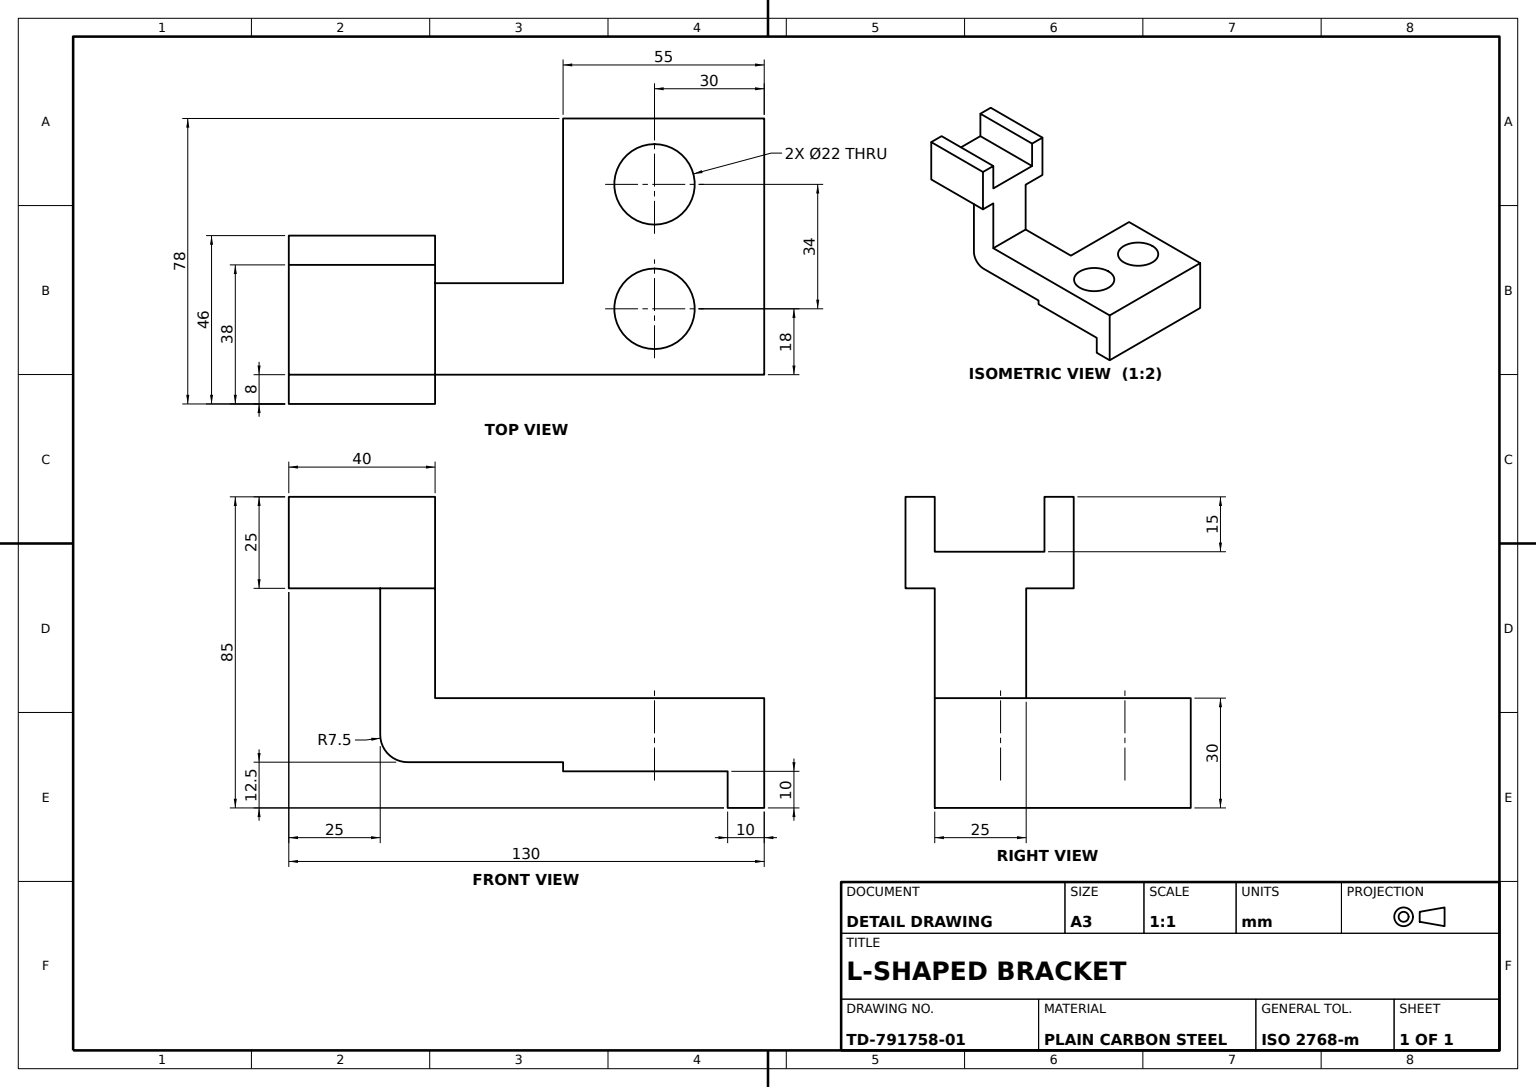
SolidWorks part; units mm, degrees
material "Plain Carbon Steel"
ref_plane "Front Plane" through (0, 0, 0) normal (0, 0, 1) x (1, 0, 0)
ref_plane "Top Plane" through (0, 0, 0) normal (0, 1, 0) x (1, 0, 0)
ref_plane "Right Plane" through (0, 0, 0) normal (1, 0, 0) x (0, 0, -1)
sketch "Base Bracket Profile Sketch" plane through (0, 0, 0) normal (0, 0, 1) x (1, 0, 0)
  line L0 (0, 0) -> (45, 0)
  line L1 (45, 0) -> (45, -10)
  line L2 (45, -10) -> (55, -10)
  line L3 (55, -10) -> (55, 20)
  line L4 (55, 20) -> (0, 20)
  line L5 (0, 20) -> (0, 0)
  dimension "D1" = 45
  dimension "D2" = 55
  dimension "D3" = 30
extrude "Base Bracket" add sketch "Base Bracket Profile Sketch" along normal blind 70
sketch "Upright Post Sketch" plane through (0, 0, 70) normal (0, 0, 1) x (1, 0, 0)
  line L0 (0, 20) -> (0, 2.5)
  line L1 (0, 20) -> (0, 0) construction
  line L2 (0, 2.5) -> (-42.5, 2.5)
  line L3 (0, 20) -> (-35, 20)
  line L4 (0, 2.5) -> (0, 10)
  line L6 (-35, 20) -> (-35, 50)
  line L7 (-35, 50) -> (-50, 50)
  line L9 (55, -10) -> (55, 20) construction
  line L10 (-50, 50) -> (-50, 10)
  line L11 (0, 0) -> (45, 0) construction
  arc A0 (-50, 10) -> (-42.5, 2.5) centre (-42.5, 10) ccw
  dimension "D1" = 15
  dimension "D2" = 105
  dimension "D3" = 7.5
  dimension "D4" = 50
extrude "Upright Post" add sketch "Upright Post Sketch" against normal blind 25 contours L10 A0 L2 L0 L3 L6 L7
sketch "Slotted Head Profile Sketch" plane through (-35, 0, 0) normal (1, 0, 0) x (0, 0, -1)
  line L0 (-70, 50) -> (-78, 50)
  line L1 (-78, 50) -> (-78, 75)
  line L2 (-78, 75) -> (-70, 75)
  line L3 (-70, 75) -> (-70, 60)
  line L4 (-70, 60) -> (-40, 60)
  line L5 (-40, 60) -> (-40, 75)
  line L6 (-40, 75) -> (-32, 75)
  line L7 (-32, 75) -> (-32, 50)
  line L8 (-32, 50) -> (-70, 50)
  line L9 (-70, 20) -> (-70, 50) construction
  line L10 (-45, 20) -> (-70, 20) construction
  dimension "D1" = 30
  dimension "D2" = 38
  dimension "D3" = 40
  dimension "D4" = 55
extrude "Slotted Head" add sketch "Slotted Head Profile Sketch" against normal blind 40
sketch "Base Holes Sketch" plane through (0, 20, 0) normal (0, 1, 0) x (1, 0, 0)
  line L0 (55, -70) -> (-35, -70) construction
  line L1 (55, 0) -> (0, 0) construction
  line L2 (55, -70) -> (55, 0) construction
  circle A0 centre (25, -18) radius 11
  circle A1 centre (25, -52) radius 11
  dimension "D1" = 22
  dimension "D2" = 22
  dimension "D7" = 22
  dimension "D3" = 18
  dimension "D4" = 18
  dimension "D5" = 34
  dimension "D6" = 30
extrude "Base Holes 2xØ22" cut sketch "Base Holes Sketch" against normal blind 30
